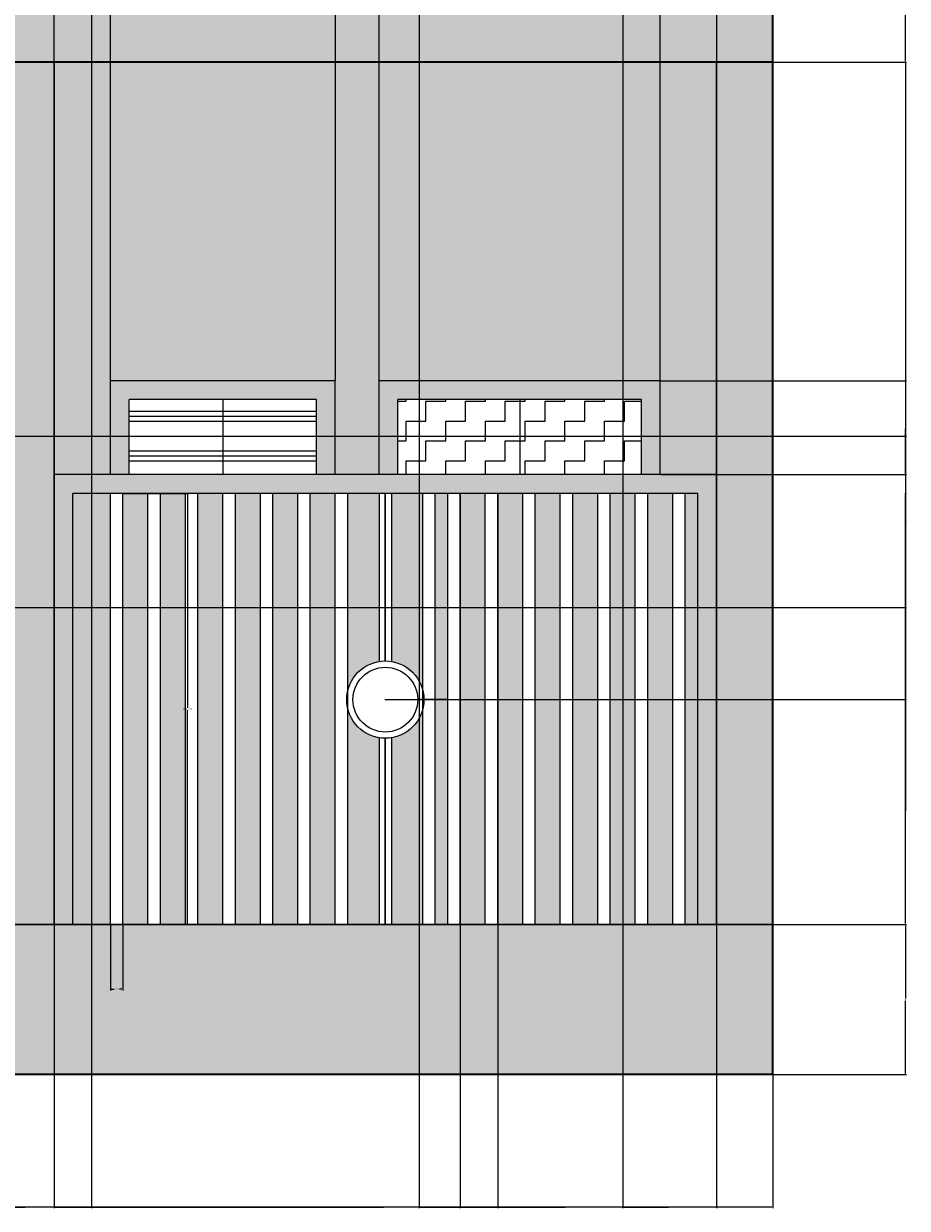
# Model space of a CAD drawing. Units: inches. Extents: x 2051 to 2334, y 814 to 1281.
# Tile 2 of 4: x 2193 to 2334, y 814 to 1003. Entities that reach past the tile are written whole.
import ezdxf

# ---------------------------------------------------------------- set-up
doc = ezdxf.new("R2010")
doc.units = ezdxf.units.IN
for name, color, linetype, lineweight in [('A-ANNO-DIMS', 2, 'Continuous', 18), ('A-COLS', 7, 'Continuous', 30), ('A-DOOR', 3, 'Continuous', 20), ('A-DOOR-GATE', 7, 'Continuous', 20), ('A-ELEV-FRAM', 7, 'Continuous', 35), ('A-ELEV-OPEN-PATT', 36, 'Continuous', 13), ('A-GLAZ', 4, 'Continuous', 18), ('A-WALL', 7, 'Continuous', 30)]:
    doc.layers.add(name, color=color, linetype=linetype, lineweight=lineweight)
for name, color, linetype, lineweight, true_color in [('A-DOOR-GATE-FRAM-PATT', 251, 'Continuous', 13, 0x636466), ('A-DOOR-GATE-PATT', 253, 'Continuous', 13, 0x9898cc), ('A-DOOR-PATT', 251, 'Continuous', 13, 0x636466), ('A-ELEV-FRAM-PATT', 251, 'Continuous', 13, 0x636466), ('A-GLAZ-SCRN-PATT', 251, 'Continuous', 13, 0x636466), ('A-WALL-PATT', 9, 'Continuous', 13, 0xc7c8ca), ('A-WALL-RECS-PATT', 61, 'Continuous', 13, 0xedee99)]:
    doc.layers.add(name, color=color, linetype=linetype, lineweight=lineweight, true_color=true_color)
doc.styles.get("Standard").update_dxf_attribs({"font": 'arial.ttf'})
doc.dimstyles.get("Standard").update_dxf_attribs({"dimtxt": 0.18, "dimasz": 0.18, "dimexe": 0.18, "dimexo": 0.0625, "dimgap": 0.09, "dimtad": 0, "dimtih": 1, "dimtoh": 1, "dimdec": 4, "dimzin": 0, "dimdsep": 46, "dimtxsty": 'Standard', "dimcen": 0.09, "dimadec": 0, "dimazin": 0, "dimtfac": 1, "dimtdec": 4, "dimtofl": 0, "dimtmove": 0, "dimatfit": 3, "dimfxl": 1, "dimtolj": 1, "dimtzin": 0, "dimarcsym": 0})

# ---------------------------------------------------------------- blocks, each defined once
blk = doc.blocks.new('GATE-STILE-2X69')
for p, q in [((0, 0), (0, 69)), ((2, 0), (2, 69))]:
    blk.add_line(p, q)
blk = doc.blocks.new('*D3')
at = {"layer": 'A-ANNO-DIMS', "color": 0, "lineweight": -2, "transparency": 16777216}
for p, q in [((2208.99, 928.24), (2219.46, 928.24)), ((2219.28, 928.06), (2219.28, 893.93)), ((2219.28, 859.42), (2219.28, 893.56)), ((2208.99, 859.24), (2219.46, 859.24))]:
    blk.add_line(p, q, dxfattribs=at)
at = {"layer": 'A-ANNO-DIMS', "color": 0, "transparency": 16777216}
for points in [[(2219.25, 928.06), (2219.31, 928.06), (2219.28, 928.24)], [(2219.25, 859.42), (2219.31, 859.42), (2219.28, 859.24)]]:
    blk.add_solid(points, dxfattribs=at)
at = {"layer": 'Defpoints', "color": 0, "transparency": 16777216}
for p in [(2208.93, 928.24), (2219.28, 928.24), (2208.93, 859.24)]:
    blk.add_point(p, dxfattribs=at)
at = {"layer": 'A-ANNO-DIMS', "color": 0, "transparency": 16777216, "insert": (2219.28, 893.74), "char_height": 0.18, "attachment_point": 5}
blk.add_mtext('\\A1;STILE 69 TYP.', dxfattribs=at)
blk = doc.blocks.new('*D4')
at = {"layer": 'A-ANNO-DIMS', "color": 0, "lineweight": -2, "transparency": 16777216}
for p, q in [((2206.93, 859.18), (2206.93, 848.71)), ((2208.93, 859.18), (2208.93, 848.71)), ((2207.11, 848.89), (2207.47, 848.89)), ((2208.75, 848.89), (2208.39, 848.89))]:
    blk.add_line(p, q, dxfattribs=at)
at = {"layer": 'A-ANNO-DIMS', "color": 0, "transparency": 16777216}
for points in [[(2207.11, 848.92), (2207.11, 848.86), (2206.93, 848.89)], [(2208.75, 848.92), (2208.75, 848.86), (2208.93, 848.89)]]:
    blk.add_solid(points, dxfattribs=at)
at = {"layer": 'Defpoints', "color": 0, "transparency": 16777216}
for p in [(2206.93, 859.24), (2208.93, 859.24), (2208.93, 848.89)]:
    blk.add_point(p, dxfattribs=at)
at = {"layer": 'A-ANNO-DIMS', "color": 0, "transparency": 16777216, "insert": (2207.93, 848.89), "char_height": 0.18, "attachment_point": 5}
blk.add_mtext('\\A1;2 TYP.', dxfattribs=at)
blk = doc.blocks.new('*D7')
at = {"layer": 'A-ANNO-DIMS', "color": 0, "lineweight": -2, "transparency": 16777216}
for p, q in [((2072.93, 835.18), (2072.93, 813.85)), ((2312.93, 835.18), (2312.93, 813.85)), ((2073.11, 814.03), (2192.64, 814.03)), ((2312.75, 814.03), (2193.22, 814.03))]:
    blk.add_line(p, q, dxfattribs=at)
at = {"layer": 'A-ANNO-DIMS', "color": 0, "transparency": 16777216}
for points in [[(2073.11, 814.06), (2073.11, 814), (2072.93, 814.03)], [(2312.75, 814.06), (2312.75, 814), (2312.93, 814.03)]]:
    blk.add_solid(points, dxfattribs=at)
at = {"layer": 'Defpoints', "color": 0, "transparency": 16777216}
for p in [(2072.93, 835.24), (2312.93, 835.24), (2312.93, 814.03)]:
    blk.add_point(p, dxfattribs=at)
at = {"layer": 'A-ANNO-DIMS', "color": 0, "transparency": 16777216, "insert": (2192.93, 814.03), "char_height": 0.18, "attachment_point": 5}
blk.add_mtext('\\A1;240', dxfattribs=at)
blk = doc.blocks.new('*D9')
at = {"layer": 'A-ANNO-DIMS', "color": 0, "lineweight": -2, "transparency": 16777216}
for p, q in [((2312.99, 859.24), (2334.32, 859.24)), ((2334.14, 859.06), (2334.14, 847.42)), ((2334.14, 835.42), (2334.14, 847.06)), ((2312.99, 835.24), (2334.32, 835.24))]:
    blk.add_line(p, q, dxfattribs=at)
at = {"layer": 'A-ANNO-DIMS', "color": 0, "transparency": 16777216}
for points in [[(2334.11, 859.06), (2334.17, 859.06), (2334.14, 859.24)], [(2334.11, 835.42), (2334.17, 835.42), (2334.14, 835.24)]]:
    blk.add_solid(points, dxfattribs=at)
at = {"layer": 'Defpoints', "color": 0, "transparency": 16777216}
for p in [(2312.93, 859.24), (2334.14, 859.24), (2312.93, 835.24)]:
    blk.add_point(p, dxfattribs=at)
at = {"layer": 'A-ANNO-DIMS', "color": 0, "transparency": 16777216, "insert": (2334.14, 847.24), "char_height": 0.18, "attachment_point": 5}
blk.add_mtext('\\A1;24', dxfattribs=at)
blk = doc.blocks.new('*D10')
at = {"layer": 'A-ANNO-DIMS', "color": 0, "lineweight": -2, "transparency": 16777216}
for p, q in [((2312.99, 997.24), (2334.32, 997.24)), ((2334.14, 997.06), (2334.14, 928.43)), ((2334.14, 859.42), (2334.14, 928.06)), ((2312.99, 859.24), (2334.32, 859.24))]:
    blk.add_line(p, q, dxfattribs=at)
at = {"layer": 'A-ANNO-DIMS', "color": 0, "transparency": 16777216}
for points in [[(2334.11, 997.06), (2334.17, 997.06), (2334.14, 997.24)], [(2334.11, 859.42), (2334.17, 859.42), (2334.14, 859.24)]]:
    blk.add_solid(points, dxfattribs=at)
at = {"layer": 'Defpoints', "color": 0, "transparency": 16777216}
for p in [(2312.93, 997.24), (2334.14, 997.24), (2312.93, 859.24)]:
    blk.add_point(p, dxfattribs=at)
at = {"layer": 'A-ANNO-DIMS', "color": 0, "transparency": 16777216, "insert": (2334.14, 928.24), "char_height": 0.18, "attachment_point": 5}
blk.add_mtext('\\A1;138', dxfattribs=at)
blk = doc.blocks.new('*D11')
at = {"layer": 'A-ANNO-DIMS', "color": 0, "lineweight": -2, "transparency": 16777216}
for p, q in [((2256.4, 1017.24), (2334.32, 1017.24)), ((2334.14, 1017.06), (2334.14, 1007.43)), ((2334.14, 997.42), (2334.14, 1007.06)), ((2312.99, 997.24), (2334.32, 997.24))]:
    blk.add_line(p, q, dxfattribs=at)
at = {"layer": 'A-ANNO-DIMS', "color": 0, "transparency": 16777216}
for points in [[(2334.11, 1017.06), (2334.17, 1017.06), (2334.14, 1017.24)], [(2334.11, 997.42), (2334.17, 997.42), (2334.14, 997.24)]]:
    blk.add_solid(points, dxfattribs=at)
at = {"layer": 'Defpoints', "color": 0, "transparency": 16777216}
for p in [(2256.33, 1017.24), (2334.14, 1017.24), (2312.93, 997.24)]:
    blk.add_point(p, dxfattribs=at)
at = {"layer": 'A-ANNO-DIMS', "color": 0, "transparency": 16777216, "insert": (2334.14, 1007.24), "char_height": 0.18, "attachment_point": 5}
blk.add_mtext('\\A1;20', dxfattribs=at)
blk = doc.blocks.new('*D22')
at = {"layer": 'A-ANNO-DIMS', "color": 0, "lineweight": -2, "transparency": 16777216}
for p, q in [((2303.93, 1059.18), (2303.93, 813.85)), ((2256.33, 1017.18), (2256.33, 813.85)), ((2256.51, 814.03), (2279.73, 814.03)), ((2303.75, 814.03), (2280.53, 814.03))]:
    blk.add_line(p, q, dxfattribs=at)
at = {"layer": 'A-ANNO-DIMS', "color": 0, "transparency": 16777216}
for points in [[(2256.51, 814.06), (2256.51, 814), (2256.33, 814.03)], [(2303.75, 814.06), (2303.75, 814), (2303.93, 814.03)]]:
    blk.add_solid(points, dxfattribs=at)
at = {"layer": 'Defpoints', "color": 0, "transparency": 16777216}
for p in [(2303.93, 1059.24), (2256.33, 1017.24), (2303.93, 814.03)]:
    blk.add_point(p, dxfattribs=at)
at = {"layer": 'A-ANNO-DIMS', "color": 0, "transparency": 16777216, "insert": (2280.13, 814.03), "char_height": 0.18, "attachment_point": 5}
blk.add_mtext('\\A1;47.59', dxfattribs=at)
blk = doc.blocks.new('*D28')
at = {"layer": 'A-ANNO-DIMS', "color": 0, "lineweight": -2, "transparency": 16777216}
for p, q in [((2203.93, 1065.18), (2203.93, 813.85)), ((2176.93, 1063.18), (2176.93, 813.85)), ((2177.11, 814.03), (2190.21, 814.03)), ((2203.75, 814.03), (2190.65, 814.03))]:
    blk.add_line(p, q, dxfattribs=at)
at = {"layer": 'A-ANNO-DIMS', "color": 0, "transparency": 16777216}
for points in [[(2177.11, 814.06), (2177.11, 814), (2176.93, 814.03)], [(2203.75, 814.06), (2203.75, 814), (2203.93, 814.03)]]:
    blk.add_solid(points, dxfattribs=at)
at = {"layer": 'Defpoints', "color": 0, "transparency": 16777216}
for p in [(2203.93, 1065.24), (2176.93, 1063.24), (2203.93, 814.03)]:
    blk.add_point(p, dxfattribs=at)
at = {"layer": 'A-ANNO-DIMS', "color": 0, "transparency": 16777216, "insert": (2190.43, 814.03), "char_height": 0.18, "attachment_point": 5}
blk.add_mtext('\\A1;27', dxfattribs=at)
blk = doc.blocks.new('*D29')
at = {"layer": 'A-ANNO-DIMS', "color": 0, "lineweight": -2, "transparency": 16777216}
for p, q in [((2203.93, 1065.18), (2203.93, 813.85)), ((2288.93, 1065.18), (2288.93, 813.85)), ((2204.11, 814.03), (2246.21, 814.03)), ((2288.75, 814.03), (2246.65, 814.03))]:
    blk.add_line(p, q, dxfattribs=at)
at = {"layer": 'A-ANNO-DIMS', "color": 0, "transparency": 16777216}
for points in [[(2204.11, 814.06), (2204.11, 814), (2203.93, 814.03)], [(2288.75, 814.06), (2288.75, 814), (2288.93, 814.03)]]:
    blk.add_solid(points, dxfattribs=at)
at = {"layer": 'Defpoints', "color": 0, "transparency": 16777216}
for p in [(2203.93, 1065.24), (2288.93, 1065.24), (2288.93, 814.03)]:
    blk.add_point(p, dxfattribs=at)
at = {"layer": 'A-ANNO-DIMS', "color": 0, "transparency": 16777216, "insert": (2246.43, 814.03), "char_height": 0.18, "attachment_point": 5}
blk.add_mtext('\\A1;85', dxfattribs=at)
blk = doc.blocks.new('*D30')
at = {"layer": 'A-ANNO-DIMS', "color": 0, "lineweight": -2, "transparency": 16777216}
for p, q in [((2288.93, 1065.18), (2288.93, 813.85)), ((2303.93, 1065.18), (2303.93, 813.85)), ((2289.11, 814.03), (2296.22, 814.03)), ((2303.75, 814.03), (2296.64, 814.03))]:
    blk.add_line(p, q, dxfattribs=at)
at = {"layer": 'A-ANNO-DIMS', "color": 0, "transparency": 16777216}
for points in [[(2289.11, 814.06), (2289.11, 814), (2288.93, 814.03)], [(2303.75, 814.06), (2303.75, 814), (2303.93, 814.03)]]:
    blk.add_solid(points, dxfattribs=at)
at = {"layer": 'Defpoints', "color": 0, "transparency": 16777216}
for p in [(2288.93, 1065.24), (2303.93, 1065.24), (2303.93, 814.03)]:
    blk.add_point(p, dxfattribs=at)
at = {"layer": 'A-ANNO-DIMS', "color": 0, "transparency": 16777216, "insert": (2296.43, 814.03), "char_height": 0.18, "attachment_point": 5}
blk.add_mtext('\\A1;15', dxfattribs=at)
blk = doc.blocks.new('*D38')
at = {"layer": 'A-ANNO-DIMS', "color": 0, "lineweight": -2, "transparency": 16777216}
for p, q in [((2188.93, 859.18), (2188.93, 813.85)), ((2197.93, 859.18), (2197.93, 813.85)), ((2189.11, 814.03), (2193.28, 814.03)), ((2197.75, 814.03), (2193.58, 814.03))]:
    blk.add_line(p, q, dxfattribs=at)
at = {"layer": 'A-ANNO-DIMS', "color": 0, "transparency": 16777216}
for points in [[(2189.11, 814.06), (2189.11, 814), (2188.93, 814.03)], [(2197.75, 814.06), (2197.75, 814), (2197.93, 814.03)]]:
    blk.add_solid(points, dxfattribs=at)
at = {"layer": 'Defpoints', "color": 0, "transparency": 16777216}
for p in [(2188.93, 859.24), (2197.93, 859.24), (2197.93, 814.03)]:
    blk.add_point(p, dxfattribs=at)
at = {"layer": 'A-ANNO-DIMS', "color": 0, "transparency": 16777216, "insert": (2193.43, 814.03), "char_height": 0.18, "attachment_point": 5}
blk.add_mtext('\\A1;9', dxfattribs=at)
blk = doc.blocks.new('*D39')
at = {"layer": 'A-ANNO-DIMS', "color": 0, "lineweight": -2, "transparency": 16777216}
for p, q in [((2197.93, 859.18), (2197.93, 813.85)), ((2303.93, 859.18), (2303.93, 813.85)), ((2198.11, 814.03), (2250.65, 814.03)), ((2303.75, 814.03), (2251.21, 814.03))]:
    blk.add_line(p, q, dxfattribs=at)
at = {"layer": 'A-ANNO-DIMS', "color": 0, "transparency": 16777216}
for points in [[(2198.11, 814.06), (2198.11, 814), (2197.93, 814.03)], [(2303.75, 814.06), (2303.75, 814), (2303.93, 814.03)]]:
    blk.add_solid(points, dxfattribs=at)
at = {"layer": 'Defpoints', "color": 0, "transparency": 16777216}
for p in [(2197.93, 859.24), (2303.93, 859.24), (2303.93, 814.03)]:
    blk.add_point(p, dxfattribs=at)
at = {"layer": 'A-ANNO-DIMS', "color": 0, "transparency": 16777216, "insert": (2250.93, 814.03), "char_height": 0.18, "attachment_point": 5}
blk.add_mtext('\\A1;106', dxfattribs=at)
blk = doc.blocks.new('*D42')
at = {"layer": 'A-ANNO-DIMS', "color": 0, "lineweight": -2, "transparency": 16777216}
for p, q in [((2153.2, 937.38), (2334.32, 937.38)), ((2334.14, 937.2), (2334.14, 923.88)), ((2334.14, 910.18), (2334.14, 923.51)), ((2188.99, 910), (2334.32, 910))]:
    blk.add_line(p, q, dxfattribs=at)
at = {"layer": 'A-ANNO-DIMS', "color": 0, "transparency": 16777216}
for points in [[(2334.11, 937.2), (2334.17, 937.2), (2334.14, 937.38)], [(2334.11, 910.18), (2334.17, 910.18), (2334.14, 910)]]:
    blk.add_solid(points, dxfattribs=at)
at = {"layer": 'Defpoints', "color": 0, "transparency": 16777216}
for p in [(2153.14, 937.38), (2334.14, 937.38), (2188.93, 910)]:
    blk.add_point(p, dxfattribs=at)
at = {"layer": 'A-ANNO-DIMS', "color": 0, "transparency": 16777216, "insert": (2334.14, 923.69), "char_height": 0.18, "attachment_point": 5}
blk.add_mtext('\\A1;27.38', dxfattribs=at)
blk = doc.blocks.new('*D46')
at = {"layer": 'A-ANNO-DIMS', "color": 0, "lineweight": -2, "transparency": 16777216}
for p, q in [((2303.99, 931.24), (2334.32, 931.24)), ((2334.14, 931.06), (2334.14, 895.42)), ((2334.14, 859.42), (2334.14, 895.06)), ((2303.99, 859.24), (2334.32, 859.24))]:
    blk.add_line(p, q, dxfattribs=at)
at = {"layer": 'A-ANNO-DIMS', "color": 0, "transparency": 16777216}
for points in [[(2334.11, 931.06), (2334.17, 931.06), (2334.14, 931.24)], [(2334.11, 859.42), (2334.17, 859.42), (2334.14, 859.24)]]:
    blk.add_solid(points, dxfattribs=at)
at = {"layer": 'Defpoints', "color": 0, "transparency": 16777216}
for p in [(2303.93, 931.24), (2334.14, 931.24), (2303.93, 859.24)]:
    blk.add_point(p, dxfattribs=at)
at = {"layer": 'A-ANNO-DIMS', "color": 0, "transparency": 16777216, "insert": (2334.14, 895.24), "char_height": 0.18, "attachment_point": 5}
blk.add_mtext('\\A1;72', dxfattribs=at)
blk = doc.blocks.new('*D47')
at = {"layer": 'A-ANNO-DIMS', "color": 0, "lineweight": -2, "transparency": 16777216}
for p, q in [((2262.93, 928.18), (2262.93, 813.85)), ((2268.93, 928.18), (2268.93, 813.85)), ((2263.11, 814.03), (2265.78, 814.03)), ((2268.75, 814.03), (2266.08, 814.03))]:
    blk.add_line(p, q, dxfattribs=at)
at = {"layer": 'A-ANNO-DIMS', "color": 0, "transparency": 16777216}
for points in [[(2263.11, 814.06), (2263.11, 814), (2262.93, 814.03)], [(2268.75, 814.06), (2268.75, 814), (2268.93, 814.03)]]:
    blk.add_solid(points, dxfattribs=at)
at = {"layer": 'Defpoints', "color": 0, "transparency": 16777216}
for p in [(2262.93, 928.24), (2268.93, 928.24), (2268.93, 814.03)]:
    blk.add_point(p, dxfattribs=at)
at = {"layer": 'A-ANNO-DIMS', "color": 0, "transparency": 16777216, "insert": (2265.93, 814.03), "char_height": 0.18, "attachment_point": 5}
blk.add_mtext('\\A1;6', dxfattribs=at)
blk = doc.blocks.new('*D48')
at = {"layer": 'A-ANNO-DIMS', "color": 0, "lineweight": -2, "transparency": 16777216}
for p, q in [((2250.99, 895.24), (2334.32, 895.24)), ((2334.14, 895.06), (2334.14, 877.43)), ((2334.14, 859.42), (2334.14, 877.06)), ((2250.99, 859.24), (2334.32, 859.24))]:
    blk.add_line(p, q, dxfattribs=at)
at = {"layer": 'A-ANNO-DIMS', "color": 0, "transparency": 16777216}
for points in [[(2334.11, 895.06), (2334.17, 895.06), (2334.14, 895.24)], [(2334.11, 859.42), (2334.17, 859.42), (2334.14, 859.24)]]:
    blk.add_solid(points, dxfattribs=at)
at = {"layer": 'Defpoints', "color": 0, "transparency": 16777216}
for p in [(2250.93, 895.24), (2334.14, 895.24), (2250.93, 859.24)]:
    blk.add_point(p, dxfattribs=at)
at = {"layer": 'A-ANNO-DIMS', "color": 0, "transparency": 16777216, "insert": (2334.14, 877.24), "char_height": 0.18, "attachment_point": 5}
blk.add_mtext('\\A1;36', dxfattribs=at)
blk = doc.blocks.new('*D49')
at = {"layer": 'A-ANNO-DIMS', "color": 0, "lineweight": -2, "transparency": 16777216}
for p, q in [((2197.93, 931.31), (2197.93, 1280.64)), ((2198.11, 1280.46), (2202.28, 1280.46)), ((2206.75, 1280.46), (2202.58, 1280.46)), ((2206.93, 946.31), (2206.93, 1280.64))]:
    blk.add_line(p, q, dxfattribs=at)
at = {"layer": 'A-ANNO-DIMS', "color": 0, "transparency": 16777216}
for points in [[(2198.11, 1280.49), (2198.11, 1280.43), (2197.93, 1280.46)], [(2206.75, 1280.49), (2206.75, 1280.43), (2206.93, 1280.46)]]:
    blk.add_solid(points, dxfattribs=at)
at = {"layer": 'Defpoints', "color": 0, "transparency": 16777216}
for p in [(2206.93, 1280.46), (2206.93, 946.24), (2197.93, 931.24)]:
    blk.add_point(p, dxfattribs=at)
at = {"layer": 'A-ANNO-DIMS', "color": 0, "transparency": 16777216, "insert": (2202.43, 1280.46), "char_height": 0.18, "attachment_point": 5}
blk.add_mtext('\\A1;9', dxfattribs=at)
blk = doc.blocks.new('*D50')
at = {"layer": 'A-ANNO-DIMS', "color": 0, "lineweight": -2, "transparency": 16777216}
for p, q in [((2206.93, 946.31), (2206.93, 1280.64)), ((2207.11, 1280.46), (2224.71, 1280.46)), ((2242.75, 1280.46), (2225.15, 1280.46)), ((2242.93, 946.31), (2242.93, 1280.64))]:
    blk.add_line(p, q, dxfattribs=at)
at = {"layer": 'A-ANNO-DIMS', "color": 0, "transparency": 16777216}
for points in [[(2207.11, 1280.49), (2207.11, 1280.43), (2206.93, 1280.46)], [(2242.75, 1280.49), (2242.75, 1280.43), (2242.93, 1280.46)]]:
    blk.add_solid(points, dxfattribs=at)
at = {"layer": 'Defpoints', "color": 0, "transparency": 16777216}
for p in [(2242.93, 1280.46), (2206.93, 946.24), (2242.93, 946.24)]:
    blk.add_point(p, dxfattribs=at)
at = {"layer": 'A-ANNO-DIMS', "color": 0, "transparency": 16777216, "insert": (2224.93, 1280.46), "char_height": 0.18, "attachment_point": 5}
blk.add_mtext('\\A1;36', dxfattribs=at)
blk = doc.blocks.new('*D51')
at = {"layer": 'A-ANNO-DIMS', "color": 0, "lineweight": -2, "transparency": 16777216}
for p, q in [((2242.93, 946.31), (2242.93, 1280.64)), ((2243.11, 1280.46), (2246.28, 1280.46)), ((2249.75, 1280.46), (2246.58, 1280.46)), ((2249.93, 946.31), (2249.93, 1280.64))]:
    blk.add_line(p, q, dxfattribs=at)
at = {"layer": 'A-ANNO-DIMS', "color": 0, "transparency": 16777216}
for points in [[(2243.11, 1280.49), (2243.11, 1280.43), (2242.93, 1280.46)], [(2249.75, 1280.49), (2249.75, 1280.43), (2249.93, 1280.46)]]:
    blk.add_solid(points, dxfattribs=at)
at = {"layer": 'Defpoints', "color": 0, "transparency": 16777216}
for p in [(2249.93, 1280.46), (2242.93, 946.24), (2249.93, 946.24)]:
    blk.add_point(p, dxfattribs=at)
at = {"layer": 'A-ANNO-DIMS', "color": 0, "transparency": 16777216, "insert": (2246.43, 1280.46), "char_height": 0.18, "attachment_point": 5}
blk.add_mtext('\\A1;7', dxfattribs=at)
blk = doc.blocks.new('*D52')
at = {"layer": 'A-ANNO-DIMS', "color": 0, "lineweight": -2, "transparency": 16777216}
for p, q in [((2249.93, 946.31), (2249.93, 1280.64)), ((2250.11, 1280.46), (2272.21, 1280.46)), ((2294.75, 1280.46), (2272.65, 1280.46)), ((2294.93, 946.31), (2294.93, 1280.64))]:
    blk.add_line(p, q, dxfattribs=at)
at = {"layer": 'A-ANNO-DIMS', "color": 0, "transparency": 16777216}
for points in [[(2250.11, 1280.49), (2250.11, 1280.43), (2249.93, 1280.46)], [(2294.75, 1280.49), (2294.75, 1280.43), (2294.93, 1280.46)]]:
    blk.add_solid(points, dxfattribs=at)
at = {"layer": 'Defpoints', "color": 0, "transparency": 16777216}
for p in [(2294.93, 1280.46), (2249.93, 946.24), (2294.93, 946.24)]:
    blk.add_point(p, dxfattribs=at)
at = {"layer": 'A-ANNO-DIMS', "color": 0, "transparency": 16777216, "insert": (2272.43, 1280.46), "char_height": 0.18, "attachment_point": 5}
blk.add_mtext('\\A1;45', dxfattribs=at)
blk = doc.blocks.new('*D53')
at = {"layer": 'A-ANNO-DIMS', "color": 0, "lineweight": -2, "transparency": 16777216}
for p, q in [((2294.99, 946.24), (2334.32, 946.24)), ((2334.14, 946.06), (2334.14, 938.93)), ((2334.14, 931.42), (2334.14, 938.56)), ((2294.99, 931.24), (2334.32, 931.24))]:
    blk.add_line(p, q, dxfattribs=at)
at = {"layer": 'A-ANNO-DIMS', "color": 0, "transparency": 16777216}
for points in [[(2334.11, 946.06), (2334.17, 946.06), (2334.14, 946.24)], [(2334.11, 931.42), (2334.17, 931.42), (2334.14, 931.24)]]:
    blk.add_solid(points, dxfattribs=at)
at = {"layer": 'Defpoints', "color": 0, "transparency": 16777216}
for p in [(2294.93, 946.24), (2334.14, 946.24), (2294.93, 931.24)]:
    blk.add_point(p, dxfattribs=at)
at = {"layer": 'A-ANNO-DIMS', "color": 0, "transparency": 16777216, "insert": (2334.14, 938.74), "char_height": 0.18, "attachment_point": 5}
blk.add_mtext('\\A1;15', dxfattribs=at)
blk = doc.blocks.new('*D63')
at = {"layer": 'A-ANNO-DIMS', "color": 0, "lineweight": -2, "transparency": 16777216}
for p, q in [((2250.84, 895.24), (2251.02, 895.24)), ((2250.93, 895.15), (2250.93, 895.33)), ((2260.82, 895.24), (2257.29, 895.24))]:
    blk.add_line(p, q, dxfattribs=at)
at = {"layer": 'A-ANNO-DIMS', "color": 0, "transparency": 16777216}
blk.add_solid([(2257.29, 895.27), (2257.29, 895.21), (2257.11, 895.24)], dxfattribs=at)
at = {"layer": 'Defpoints', "color": 0, "transparency": 16777216}
for p in [(2244.74, 895.24), (2257.11, 895.24)]:
    blk.add_point(p, dxfattribs=at)
at = {"layer": 'A-ANNO-DIMS', "color": 0, "transparency": 16777216, "insert": (2261.32, 895.24), "char_height": 0.18, "attachment_point": 5}
blk.add_mtext('\\A1;∅12.37', dxfattribs=at)
blk = doc.blocks.new('*D64')
at = {"layer": 'A-ANNO-DIMS', "color": 0, "lineweight": -2, "transparency": 16777216}
for p, q in [((2250.84, 895.24), (2251.02, 895.24)), ((2250.93, 895.15), (2250.93, 895.33)), ((2259.22, 895.24), (2256.29, 895.24))]:
    blk.add_line(p, q, dxfattribs=at)
at = {"layer": 'A-ANNO-DIMS', "color": 0, "transparency": 16777216}
blk.add_solid([(2256.29, 895.27), (2256.29, 895.21), (2256.11, 895.24)], dxfattribs=at)
at = {"layer": 'Defpoints', "color": 0, "transparency": 16777216}
for p in [(2245.74, 895.24), (2256.11, 895.24)]:
    blk.add_point(p, dxfattribs=at)
at = {"layer": 'A-ANNO-DIMS', "color": 0, "transparency": 16777216, "insert": (2259.72, 895.24), "char_height": 0.18, "attachment_point": 5}
blk.add_mtext('\\A1;∅10.37', dxfattribs=at)

msp = doc.modelspace()

# ---------------------------------------------------------------- hatches: boundary and pattern name
at = {"layer": 'A-DOOR-GATE-FRAM-PATT', "transparency": 33554597}
h = msp.add_hatch(color=256, dxfattribs=at)
h.dxf.hatch_style = 1
h.paths.add_polyline_path([(2303.9283, 931.2439), (2197.9283, 931.2439), (2197.9283, 859.2439), (2200.9283, 859.2439), (2200.9283, 928.2439), (2300.9283, 928.2439), (2300.9283, 859.2439), (2303.9283, 859.2439)])
at = {"layer": 'A-DOOR-GATE-PATT', "transparency": 33554597}
h = msp.add_hatch(color=256, dxfattribs=at)
h.dxf.hatch_style = 1
h.paths.add_polyline_path([(2206.9283, 928.2439), (2200.9283, 928.2439), (2200.9283, 859.2439), (2206.9283, 859.2439)])
h.paths.add_polyline_path([(2212.9283, 928.2439), (2208.9283, 928.2439), (2208.9283, 859.2439), (2212.9283, 859.2439)])
h.paths.add_polyline_path([(2218.9283, 928.2439), (2214.9283, 928.2439), (2214.9283, 859.2439), (2218.9283, 859.2439)])
h.paths.add_polyline_path([(2224.9283, 928.2439), (2220.9283, 928.2439), (2220.9283, 859.2439), (2224.9283, 859.2439)])
h.paths.add_polyline_path([(2230.9283, 928.2439), (2226.9283, 928.2439), (2226.9283, 859.2439), (2230.9283, 859.2439)])
h.paths.add_polyline_path([(2236.9283, 928.2439), (2232.9283, 928.2439), (2232.9283, 859.2439), (2236.9283, 859.2439)])
h.paths.add_polyline_path([(2242.9283, 928.2439), (2238.9283, 928.2439), (2238.9283, 859.2439), (2242.9283, 859.2439)])
h.paths.add_polyline_path([(2249.9283, 928.2439), (2244.9283, 928.2439), (2244.9283, 896.7439, -0.29934261), (2249.9283, 901.3472)])
h.paths.add_polyline_path([(2249.9283, 889.1406, -0.29934261), (2244.9283, 893.7439), (2244.9283, 859.2439), (2249.9283, 859.2439)])
h.paths.add_polyline_path([(2256.9283, 893.7439, -0.29934261), (2251.9283, 889.1406), (2251.9283, 859.2439), (2256.9283, 859.2439)])
h.paths.add_polyline_path([(2256.9283, 928.2439), (2251.9283, 928.2439), (2251.9283, 901.3472, -0.29934261), (2256.9283, 896.7439)])
h.paths.add_polyline_path([(2266.9283, 928.2439), (2262.9283, 928.2439), (2262.9283, 859.2439), (2266.9283, 859.2439)])
h.paths.add_polyline_path([(2272.9283, 928.2439), (2268.9283, 928.2439), (2268.9283, 859.2439), (2272.9283, 859.2439)])
h.paths.add_polyline_path([(2278.9283, 928.2439), (2274.9283, 928.2439), (2274.9283, 859.2439), (2278.9283, 859.2439)])
h.paths.add_polyline_path([(2284.9283, 928.2439), (2280.9283, 928.2439), (2280.9283, 859.2439), (2284.9283, 859.2439)])
h.paths.add_polyline_path([(2290.9283, 928.2439), (2286.9283, 928.2439), (2286.9283, 859.2439), (2290.9283, 859.2439)])
h.paths.add_polyline_path([(2296.9283, 928.2439), (2292.9283, 928.2439), (2292.9283, 859.2439), (2296.9283, 859.2439)])
h = msp.add_hatch(color=256, dxfattribs=at)
h.dxf.hatch_style = 1
h.paths.add_polyline_path([(2260.9283, 928.2439), (2258.9283, 928.2439), (2258.9283, 859.2439), (2260.9283, 859.2439)])
h = msp.add_hatch(color=256, dxfattribs=at)
h.dxf.hatch_style = 1
h.paths.add_polyline_path([(2300.9283, 928.2439), (2298.9283, 928.2439), (2298.9283, 859.2439), (2300.9283, 859.2439)])
at = {"layer": 'A-DOOR-PATT', "transparency": 33554595}
h = msp.add_hatch(dxfattribs=at)
h.set_pattern_fill('ZIGZAG', color=256)
h.set_pattern_definition([(0, (0, 0), (3.175, 3.175), [3.175, -3.175]), (90, (3.175, 0), (-3.175, 3.175), [3.175, -3.175])])
h.paths.add_polyline_path([(2285.9283, 1122.9709, 0.05319425), (2284.4701, 1131.2439), (2268.9283, 1131.2439), (2268.9283, 1065.2439), (2285.9283, 1065.2439)])
h.paths.add_polyline_path([(2268.9283, 1131.2439), (2250.9283, 1131.2439), (2250.9283, 1065.2439), (2268.9283, 1065.2439)])
h.paths.add_polyline_path([(2272.4283, 943.2439), (2252.9283, 943.2439), (2252.9283, 931.2439), (2272.4283, 931.2439)])
h.paths.add_polyline_path([(2291.9283, 943.2439), (2272.4283, 943.2439), (2272.4283, 931.2439), (2291.9283, 931.2439)])
at = {"layer": 'A-ELEV-FRAM-PATT'}
h = msp.add_hatch(color=256, dxfattribs=at)
h.dxf.hatch_style = 1
h.paths.add_polyline_path([(2312.9283, 1217.2439), (2303.9283, 1217.2439), (2303.9283, 1059.2439, -0.29083376), (2256.3338, 1017.2439), (2110.9283, 1017.2439, -0.41949346), (2084.9283, 1039.0559), (2084.9283, 1221.9535, -0.37464242), (2110.9283, 1247.2439), (2247.6639, 1247.2439), (2247.6639, 1259.2439), (2072.9283, 1259.2439), (2072.9283, 835.2439), (2084.9283, 835.2439), (2084.9283, 967.2832, -0.36016597), (2115.4224, 997.2439), (2312.9283, 997.2439)])
h = msp.add_hatch(color=256, dxfattribs=at)
h.dxf.hatch_style = 1
h.paths.add_polyline_path([(2312.9283, 997.2439), (2303.9283, 997.2439), (2303.9283, 859.2439), (2312.9283, 859.2439)])
h.paths.add_polyline_path([(2197.9283, 997.2439), (2188.9283, 997.2439), (2188.9283, 859.2439), (2197.9283, 859.2439)])
h = msp.add_hatch(color=256, dxfattribs=at)
h.dxf.hatch_style = 1
h.paths.add_polyline_path([(2312.9283, 859.2439), (2084.9283, 859.2439), (2084.9283, 835.2439), (2312.9283, 835.2439)])
at = {"layer": 'A-ELEV-OPEN-PATT'}
h = msp.add_hatch(color=256, dxfattribs=at)
h.dxf.hatch_style = 1
h.paths.add_polyline_path([(2227.9283, 1135.2439), (2209.7757, 1135.2439, 0.02675663), (2208.3865, 1131.2439), (2223.9283, 1131.2439), (2223.9283, 1065.2439), (2227.9283, 1065.2439)])
h.paths.add_polyline_path([(2250.9283, 1131.2439), (2284.4701, 1131.2439, 0.02675663), (2283.0809, 1135.2439), (2246.9283, 1135.2439), (2246.9283, 1065.2439), (2250.9283, 1065.2439)])
h.paths.add_polyline_path([(2242.9283, 946.2439), (2206.9283, 946.2439), (2206.9283, 931.2439), (2209.9283, 931.2439), (2209.9283, 943.2439), (2239.9283, 943.2439), (2239.9283, 931.2439), (2242.9283, 931.2439)])
h.paths.add_polyline_path([(2252.9283, 943.2439), (2291.9283, 943.2439), (2291.9283, 931.2439), (2294.9283, 931.2439), (2294.9283, 946.2439), (2249.9283, 946.2439), (2249.9283, 931.2439), (2252.9283, 931.2439)])
at = {"layer": 'A-GLAZ-SCRN-PATT', "transparency": 33554595}
h = msp.add_hatch(dxfattribs=at)
h.set_pattern_fill('PLASTI', color=256)
h.paths.add_polyline_path([(2223.9283, 1131.2439), (2208.3865, 1131.2439, 0.05319425), (2206.9283, 1122.9709), (2206.9283, 1065.2439), (2223.9283, 1065.2439)])
h.paths.add_polyline_path([(2239.9283, 943.2439), (2224.9283, 943.2439), (2224.9283, 931.2439), (2239.9283, 931.2439)])
h.paths.add_polyline_path([(2224.9283, 943.2439), (2209.9283, 943.2439), (2209.9283, 931.2439), (2224.9283, 931.2439)])
at = {"layer": 'A-WALL-PATT'}
h = msp.add_hatch(color=256, dxfattribs=at)
h.dxf.hatch_style = 1
h.paths.add_polyline_path([(2188.9283, 910.0037, 0.33864929), (2153.1397, 937.3832), (2125.034, 937.3832), (2125.034, 859.2439), (2188.9283, 859.2439)])
h.paths.add_polyline_path([(2113.034, 937.3832), (2084.9283, 937.3832), (2084.9283, 859.2439), (2113.034, 859.2439)])
h.paths.add_polyline_path([(2312.9283, 859.2439), (2084.9283, 859.2439), (2084.9283, 835.2439), (2312.9283, 835.2439)])
h.paths.add_polyline_path([(2288.9283, 1123.0714), (2288.9283, 1065.2439), (2303.9283, 1065.2439), (2303.9283, 1175.2439), (2176.9283, 1175.2439), (2176.9283, 1065.2439), (2203.9283, 1065.2439), (2203.9283, 1123.0714, -0.93632991)])
h.paths.add_polyline_path([(2197.9283, 1247.2439), (2112.9283, 1247.2439), (2112.9283, 1217.2439), (2197.9283, 1217.2439)])
h.paths.add_polyline_path([(2110.9283, 1247.2439, 0.11468321), (2098.9283, 1243.754), (2098.9283, 1019.2065, 0.12996728), (2110.9283, 1017.2439)])
h.paths.add_polyline_path([(2096.9283, 1242.5167, 0.22673474), (2084.9283, 1221.9535), (2084.9283, 1039.0559, 0.24937907), (2096.9283, 1020.2168)])
at = {"layer": 'A-WALL-RECS-PATT'}
h = msp.add_hatch(color=256, dxfattribs=at)
h.dxf.hatch_style = 1
h.paths.add_polyline_path([(2303.9283, 997.2439), (2197.9283, 997.2439), (2197.9283, 931.2439), (2206.9283, 931.2439), (2206.9283, 946.2439), (2242.9283, 946.2439), (2242.9283, 931.2439), (2249.9283, 931.2439), (2249.9283, 946.2439), (2252.9283, 946.2439), (2294.9283, 946.2439), (2294.9283, 931.2439), (2303.9283, 931.2439)])

# ---------------------------------------------------------------- linework, layer by layer
at = {"layer": 'A-COLS'}
for p, q in [((2197.9283, 859.2439), (2197.9283, 997.2439)), ((2303.9283, 859.2439), (2303.9283, 997.2439))]:
    msp.add_line(p, q, dxfattribs=at)
at = {"layer": 'A-DOOR'}
for p, q in [((2294.9283, 946.2439), (2249.9283, 946.2439)), ((2249.9283, 931.2439), (2249.9283, 946.2439)), ((2252.9283, 946.2439), (2249.9283, 946.2439)), ((2294.9283, 931.2439), (2294.9283, 946.2439)), ((2291.9283, 943.2439), (2252.9283, 943.2439)), ((2252.9283, 931.2439), (2252.9283, 943.2439)), ((2272.4283, 943.2439), (2272.4283, 931.2439)), ((2291.9283, 931.2439), (2291.9283, 943.2439))]:
    msp.add_line(p, q, dxfattribs=at)
at = {"layer": 'A-DOOR-GATE'}
for p, q in [((2303.9283, 931.2439), (2197.9283, 931.2439)), ((2300.9283, 928.2439), (2200.9283, 928.2439)), ((2200.9283, 859.2439), (2200.9283, 928.2439)), ((2249.9283, 928.2439), (2249.9283, 901.4286)), ((2250.9283, 928.2439), (2250.9283, 901.4286)), ((2250.9283, 928.2439), (2250.9283, 901.4286)), ((2250.9283, 901.4286), (2250.9283, 928.2439)), ((2251.9283, 928.2439), (2251.9283, 901.3472)), ((2300.9283, 859.2439), (2300.9283, 928.2439)), ((2249.9283, 889.0592), (2249.9283, 859.2439)), ((2250.9283, 859.2439), (2250.9283, 889.0592)), ((2250.9283, 889.0592), (2250.9283, 859.2439)), ((2250.9283, 889.0592), (2250.9283, 859.2439)), ((2251.9283, 889.1406), (2251.9283, 859.2439))]:
    msp.add_line(p, q, dxfattribs=at)
for radius in [6.1847, 5.1847]:
    msp.add_circle((2250.9283, 895.2439), radius, dxfattribs=at)
at = {"layer": 'A-ELEV-FRAM'}
for p, q in [((2312.9283, 835.2439), (2312.9283, 1217.2439)), ((2312.9283, 997.2439), (2115.4224, 997.2439)), ((2312.9283, 835.2439), (2072.9283, 835.2439))]:
    msp.add_line(p, q, dxfattribs=at)
at = {"layer": 'A-GLAZ'}
for p, q in [((2242.9283, 946.2439), (2206.9283, 946.2439)), ((2206.9283, 931.2439), (2206.9283, 946.2439)), ((2242.9283, 931.2439), (2242.9283, 946.2439)), ((2239.9283, 943.2439), (2209.9283, 943.2439)), ((2209.9283, 931.2439), (2209.9283, 943.2439)), ((2224.9283, 943.2439), (2224.9283, 931.2439)), ((2239.9283, 931.2439), (2239.9283, 943.2439))]:
    msp.add_line(p, q, dxfattribs=at)
at = {"layer": 'A-WALL'}
msp.add_line((2312.9283, 859.2439), (2084.9283, 859.2439), dxfattribs=at)

# ---------------------------------------------------------------- block references
at = {"layer": 'A-DOOR-GATE'}
for p in [(2206.9283, 859.2439), (2212.9283, 859.2439), (2218.9283, 859.2439), (2224.9283, 859.2439), (2230.9283, 859.2439), (2236.9283, 859.2439), (2242.9283, 859.2439), (2256.9283, 859.2439), (2260.9283, 859.2439), (2266.9283, 859.2439), (2272.9283, 859.2439), (2278.9283, 859.2439), (2284.9283, 859.2439), (2290.9283, 859.2439), (2296.9283, 859.2439)]:
    msp.add_blockref('GATE-STILE-2X69', p, dxfattribs=at)

# ---------------------------------------------------------------- dimensions: what is measured, and where the dimension line sits
at = {"layer": 'A-ANNO-DIMS'}
for base, p1, p2, override, picture, middle in [((2206.9283, 1280.4589), (2197.9283, 931.2439), (2206.9283, 946.2439), {"dimdec": 0, "dimlfac": 1, "dimrnd": 0, "dimzin": 0, "dimdsep": 46, "dimlunit": 2}, '*D49', (2202.4283, 1280.4589)), ((2242.9283, 1280.4589), (2206.9283, 946.2439), (2242.9283, 946.2439), {"dimdec": 0, "dimlfac": 1, "dimrnd": 0, "dimzin": 0, "dimdsep": 46, "dimlunit": 2}, '*D50', (2224.9283, 1280.4589)), ((2249.9283, 1280.4589), (2242.9283, 946.2439), (2249.9283, 946.2439), {"dimdec": 0, "dimlfac": 1, "dimrnd": 0, "dimzin": 0, "dimdsep": 46, "dimlunit": 2}, '*D51', (2246.4283, 1280.4589)), ((2294.9283, 1280.4589), (2249.9283, 946.2439), (2294.9283, 946.2439), {"dimdec": 0, "dimlfac": 1, "dimrnd": 0, "dimzin": 0, "dimdsep": 46, "dimlunit": 2}, '*D52', (2272.4283, 1280.4589)), ((2203.9283, 814.0289), (2176.9283, 1063.2439), (2203.9283, 1065.2439), {"dimdec": 0, "dimlfac": 1, "dimrnd": 0, "dimzin": 0, "dimdsep": 46, "dimlunit": 2}, '*D28', (2190.4283, 814.0289)), ((2288.9283, 814.0289), (2203.9283, 1065.2439), (2288.9283, 1065.2439), {"dimdec": 0, "dimlfac": 1, "dimrnd": 0, "dimzin": 0, "dimdsep": 46, "dimlunit": 2}, '*D29', (2246.4283, 814.0289)), ((2303.9283, 814.0289), (2288.9283, 1065.2439), (2303.9283, 1065.2439), {"dimdec": 0, "dimlfac": 1, "dimrnd": 0, "dimzin": 0, "dimdsep": 46, "dimlunit": 2}, '*D30', (2296.4283, 814.0289)), ((2303.9283, 814.0289), (2256.3338, 1017.2439), (2303.9283, 1059.2439), {"dimdec": 2, "dimlfac": 1, "dimrnd": 0, "dimzin": 0, "dimdsep": 46, "dimlunit": 2}, '*D22', (2280.131, 814.0289)), ((2268.9283, 814.0289), (2262.9283, 928.2439), (2268.9283, 928.2439), {"dimdec": 0, "dimlfac": 1, "dimrnd": 0, "dimzin": 0, "dimdsep": 46, "dimlunit": 2}, '*D47', (2265.9283, 814.0289)), ((2197.9283, 814.0289), (2188.9283, 859.2439), (2197.9283, 859.2439), {"dimdec": 0, "dimlfac": 1, "dimrnd": 0, "dimzin": 0, "dimdsep": 46, "dimlunit": 2}, '*D38', (2193.4283, 814.0289)), ((2303.9283, 814.0289), (2197.9283, 859.2439), (2303.9283, 859.2439), {"dimdec": 0, "dimlfac": 1, "dimrnd": 0, "dimzin": 0, "dimdsep": 46, "dimlunit": 2}, '*D39', (2250.9283, 814.0289)), ((2312.9283, 814.0289), (2072.9283, 835.2439), (2312.9283, 835.2439), {"dimdec": 0, "dimlfac": 1, "dimrnd": 0, "dimzin": 0, "dimdsep": 46, "dimlunit": 2}, '*D7', (2192.9283, 814.0289))]:
    dim = msp.add_linear_dim(base=base, p1=p1, p2=p2, dimstyle='Standard', override=override, dxfattribs=at)
    dim.commit()
    dim.dimension.update_dxf_attribs({"geometry": picture, "text_midpoint": middle})
for base, p1, p2, override, picture, middle in [((2334.1433, 1017.2439), (2312.9283, 997.2439), (2256.3338, 1017.2439), {"dimdec": 0, "dimlfac": 1, "dimrnd": 0, "dimzin": 0, "dimdsep": 46, "dimlunit": 2}, '*D11', (2334.1433, 1007.2439)), ((2334.1433, 997.2439), (2312.9283, 859.2439), (2312.9283, 997.2439), {"dimdec": 0, "dimlfac": 1, "dimrnd": 0, "dimzin": 0, "dimdsep": 46, "dimlunit": 2}, '*D10', (2334.1433, 928.2439)), ((2334.1433, 946.2439), (2294.9283, 931.2439), (2294.9283, 946.2439), {"dimdec": 0, "dimlfac": 1, "dimrnd": 0, "dimzin": 0, "dimdsep": 46, "dimlunit": 2}, '*D53', (2334.1433, 938.7439)), ((2334.1433, 937.3832), (2188.9283, 910.0037), (2153.1397, 937.3832), {"dimdec": 2, "dimlfac": 1, "dimrnd": 0, "dimzin": 0, "dimdsep": 46, "dimlunit": 2}, '*D42', (2334.1433, 923.6934)), ((2334.1433, 931.2439), (2303.9283, 859.2439), (2303.9283, 931.2439), {"dimdec": 0, "dimlfac": 1, "dimrnd": 0, "dimzin": 0, "dimdsep": 46, "dimlunit": 2}, '*D46', (2334.1433, 895.2439)), ((2334.1433, 895.2439), (2250.9283, 859.2439), (2250.9283, 895.2439), {"dimdec": 0, "dimlfac": 1, "dimrnd": 0, "dimzin": 0, "dimdsep": 46, "dimlunit": 2}, '*D48', (2334.1433, 877.2439)), ((2334.1433, 859.2439), (2312.9283, 835.2439), (2312.9283, 859.2439), {"dimdec": 0, "dimlfac": 1, "dimrnd": 0, "dimzin": 0, "dimdsep": 46, "dimlunit": 2}, '*D9', (2334.1433, 847.2439))]:
    dim = msp.add_linear_dim(base=base, p1=p1, p2=p2, angle=90, dimstyle='Standard', override=override, dxfattribs=at)
    dim.commit()
    dim.dimension.update_dxf_attribs({"geometry": picture, "text_midpoint": middle})
dim = msp.add_linear_dim(base=(2219.2783, 928.2439), p1=(2208.9283, 859.2439), p2=(2208.9283, 928.2439), angle=90, text='STILE <> TYP.', dimstyle='Standard', override={"dimdec": 0, "dimlfac": 1, "dimrnd": 0, "dimzin": 0, "dimdsep": 46, "dimlunit": 2}, dxfattribs=at)
dim.commit()
dim.dimension.update_dxf_attribs({"geometry": '*D3', "text_midpoint": (2219.2783, 893.7439)})
for p1, p2, picture, middle in [((2244.7436, 895.2438), (2257.113, 895.244), '*D63', (2260.8238, 895.2441)), ((2245.7436, 895.2438), (2256.113, 895.244), '*D64', (2259.2238, 895.2441))]:
    dim = msp.add_diameter_dim_2p(p1=p1, p2=p2, dimstyle='Standard', override={"dimdec": 2, "dimlfac": 1, "dimrnd": 0, "dimzin": 0, "dimdsep": 46, "dimlunit": 2}, dxfattribs=at)
    dim.commit()
    dim.dimension.update_dxf_attribs({"geometry": picture, "text_midpoint": middle, "dimtype": 163})
dim = msp.add_linear_dim(base=(2208.9283, 848.8939), p1=(2206.9283, 859.2439), p2=(2208.9283, 859.2439), text='<> TYP.', dimstyle='Standard', override={"dimdec": 0, "dimlfac": 1, "dimrnd": 0, "dimzin": 0, "dimdsep": 46, "dimlunit": 2}, dxfattribs=at)
dim.commit()
dim.dimension.update_dxf_attribs({"geometry": '*D4', "text_midpoint": (2207.9283, 848.8939)})

doc.saveas('drawing.dxf')
